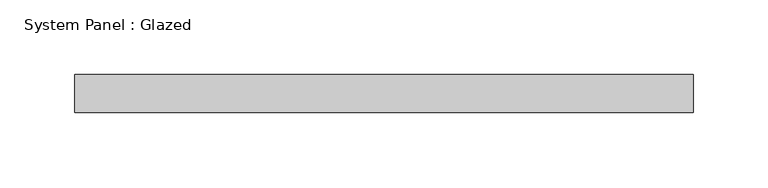
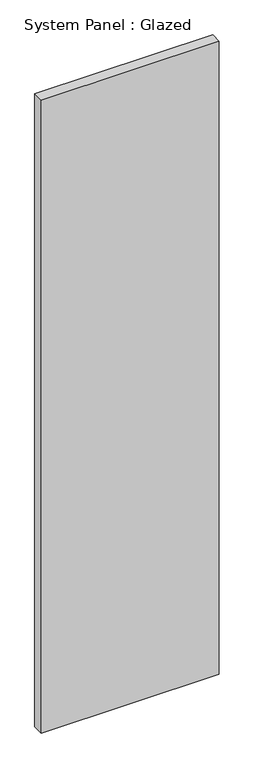
"""IFC4 building model written with IfcOpenShell, lengths in millimetres: plate geometry, System Panel : Glazed."""

from ifc_helpers import new_model, si_unit, origin, origin_with_axes, place, context, project, spatial, polyline, outline, extrude, source, transform, mapped, element, save


def system_panel_glazed_5edd0c1a(model_context):
    return source(origin(), model_context, "Body", "SweptSolid", [
        extrude(outline(polyline([(206.375, 19.05), (-206.375, 19.05), (-206.375, 44.45), (206.375, 44.45), (206.375, 19.05)])), origin_with_axes(), (0.0, 0.0, 1.0), 1550.4900448),
    ])


if __name__ == "__main__":
    model = new_model("IFC4")
    model_context = context("Model", 3, world=origin())
    ifc_project = project(units=[si_unit("LENGTHUNIT", "METRE", prefix="MILLI")], contexts=[model_context])
    site = spatial("IfcSite", under=ifc_project)
    building = spatial("IfcBuilding", under=site)
    placement = place(None, origin())
    system_panel_glazed_shape = system_panel_glazed_5edd0c1a(model_context)
    element("IfcPlate", 1, ObjectType="System Panel : Glazed", at=placement, inside=building, context=model_context, shape_type="MappedRepresentation", body=[
        mapped(system_panel_glazed_shape, transform((0.0, 0.0, 0.0), x_axis=(1.0, 0.0, 0.0), y_axis=(0.0, 1.0, 0.0), z_axis=(0.0, 0.0, 1.0))),
    ])
    save(model, "model.ifc")

# Revit data of these elements
# Type "System Panel : Glazed"
#   Construction Type Id = "GSP4R"
#   Analytic Construction = "1/8 in Pilkington single glazing"
#   Visual Light Transmittance = 0.9
#   Solar Heat Gain Coefficient = 0.86
#   Heat Transfer Coefficient (U) = 1.18115 BTU/(h·ft²·°F)
#   Define Thermal Properties by = 1
# Element 1 (IfcPlate, "System Panel : Glazed")
#   Materials on its faces: "Glass"
# Materials
#   "Glass": class "Glass", colour RGB 0 128 192, transparency 0.75, Description = "Soda Lime Glass", Cost = 0
